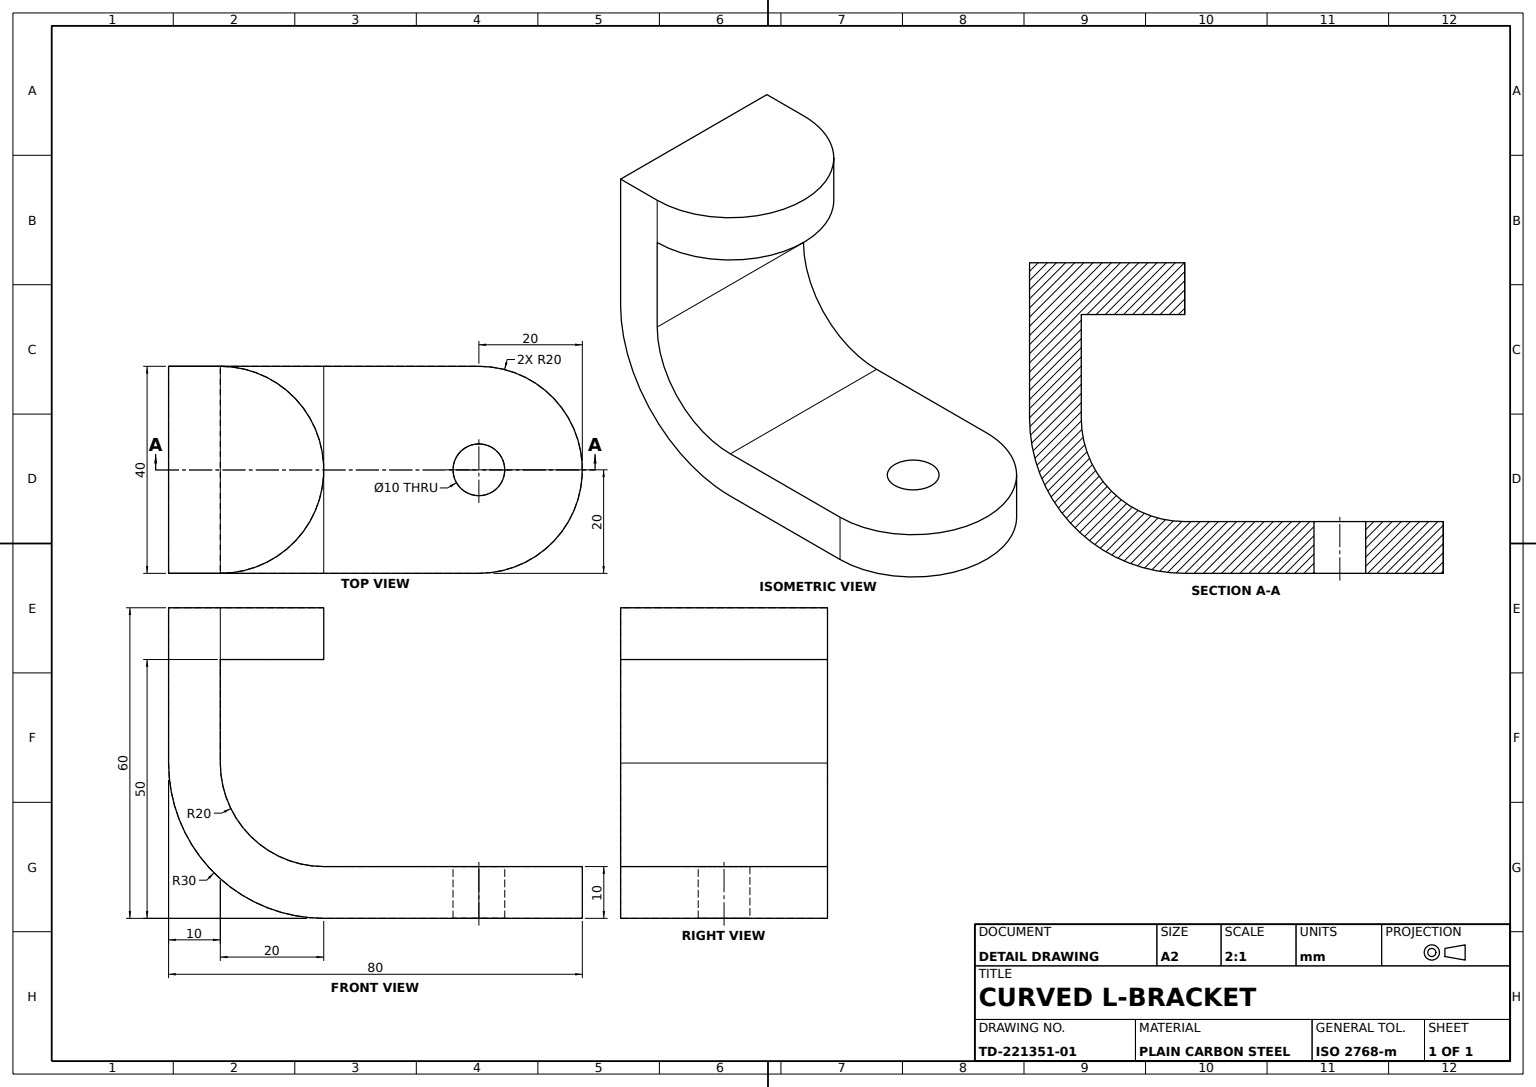
SolidWorks part; units mm, degrees
material "Plain Carbon Steel"
ref_plane "Front Plane" through (0, 0, 0) normal (0, 0, 1) x (1, 0, 0)
ref_plane "Top Plane" through (0, 0, 0) normal (0, 1, 0) x (1, 0, 0)
ref_plane "Right Plane" through (0, 0, 0) normal (1, 0, 0) x (0, 0, -1)
sketch "Bracket Profile Sketch" plane through (0, 0, 0) normal (0, 0, 1) x (1, 0, 0)
  line L0 (0, 20) -> (0, 50)
  line L1 (20, 0) -> (50, 0)
  arc A0 (20, 0) -> (0, 20) centre (20, 20) cw
  point P6 (0, 0)
  dimension "D1" = 20
  dimension "D2" = 50
extrude "Curved Bracket Wall" add sketch "Bracket Profile Sketch" along normal blind 40 thin thin type one direction wall 10
sketch "Rounded Tab Sketch" plane through (0, 50, 0) normal (0, 1, 0) x (1, 0, 0)
  line L0 (0, -40) -> (0, 0) construction
  line L1 (0, 0) -> (0, -40)
  arc A0 (0, -40) -> (0, 0) centre (0, -20) ccw
extrude "Rounded End Tab" add sketch "Rounded Tab Sketch" against normal blind 10
ref_plane "Mounting Tab Plane" through (0, 0, 0) normal (0, 1, 0) x (1, 0, 0)
sketch "Mounting Tab Sketch" plane through (0, 0, 0) normal (0, 1, 0) x (1, 0, 0)
  line L0 (50, -40) -> (50, 0) construction
  line L1 (50, 0) -> (50, -40)
  arc A0 (50, -40) -> (50, 0) centre (50, -20) ccw
extrude "Mounting Tab" add sketch "Mounting Tab Sketch" against normal blind 10
sketch "Mounting Hole Sketch" plane through (0, 0, 0) normal (0, 1, 0) x (1, 0, 0)
  circle A0 centre (50, -20) radius 5
  dimension "D1" = 10
extrude "Mounting Hole Ø10" cut sketch "Mounting Hole Sketch" against normal blind 10
